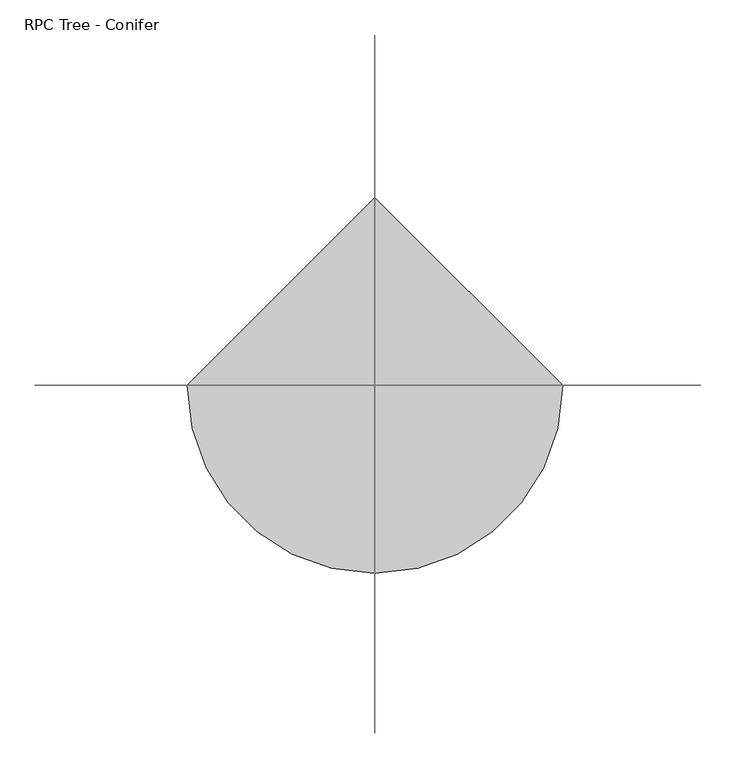
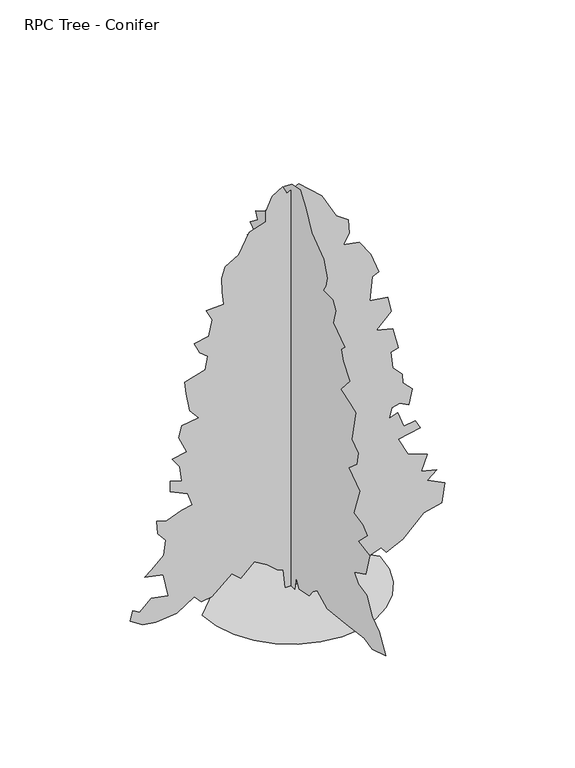
"""IFC4 building model written with IfcOpenShell, lengths in millimetres: geographic element geometry, RPC Tree - Conifer."""

from ifc_helpers import new_model, si_unit, origin, place, context, project, spatial, triangles, source, transform, mapped, element, save


def rpc_tree_conifer_9825e489(model_context):
    return source(origin(), model_context, "Body", "Tessellation", [
        triangles([(0.1966736, 56.9494036, 4.14e-05), (0.1966822, 87.893554, 239.8173931), (0.1966871, 126.5738239, 348.1206479), (0.196691, 265.8223646, 270.7615617), (0.1966966, 436.0144835, 201.1371414), (0.1967043, 629.4157963, 170.192991), (0.1967132, 823.3543219, 178.424865), (0.1967103, 846.0257578, 46.416371), (0.1967193, 985.2745983, 139.2488314), (0.196723, 1133.0273529, 41.5309043), (0.1967288, 1240.5636669, 77.3605215), (0.1967379, 1449.4382721, 69.6244157), (0.1967452, 1550.0050987, 162.4568716), (0.1967611, 1766.6151329, 371.3292603), (0.1967571, 1635.1015034, 433.2170162), (0.1967531, 1519.061348, 471.8989938), (0.1967479, 1410.9707073, 462.869276), (0.1967506, 1387.5477184, 587.9391855), (0.1967552, 1418.4916145, 696.2441299), (0.1967638, 1526.7964863, 820.0196417), (0.1967596, 1418.4916145, 843.2282541), (0.1967657, 1503.5878738, 920.5893751), (0.196761, 1372.0771511, 959.2684822), (0.1967569, 1232.8283833, 1028.8943195), (0.1967579, 1161.2365322, 1172.1522177), (0.1967675, 1341.1334003, 1222.2955959), (0.196773, 1418.4916145, 1291.9186718), (0.1967692, 1317.9247879, 1315.1272842), (0.1967646, 1147.7320513, 1415.6968723), (0.196772, 1271.5074177, 1477.5846645), (0.1967785, 1281.5201786, 1681.3043518), (0.1967728, 1139.9939335, 1701.929837), (0.1967682, 1016.2184217, 1732.8737331), (0.1967732, 1034.477845, 1873.8285015), (0.1967812, 1185.2224228, 1916.3224194), (0.196787, 1217.3549818, 2065.5239227), (0.1967808, 1093.5795427, 2042.3153103), (0.1967818, 1015.412657, 2192.8769051), (0.1967888, 1101.3147537, 2297.6043789), (0.1967867, 993.0098093, 2390.4359219), (0.1967939, 1101.3147537, 2467.7970428), (0.1967971, 1132.2586498, 2529.6848351), (0.1967921, 938.8573734, 2653.4630356), (0.1967934, 915.648761, 2730.8213951), (0.1968026, 1070.3709303, 2808.1823708), (0.1968025, 1000.745093, 2908.7634407), (0.1967977, 846.0257578, 2978.3722733), (0.1968056, 946.5925844, 3094.4151901), (0.1968038, 838.28764, 3194.9706802), (0.1968006, 699.0416336, 3295.554657), (0.1968039, 691.3035158, 3419.3415779), (0.1968107, 807.3437439, 3473.4911797), (0.1968087, 722.250246, 3535.3847855), (0.1968049, 621.6805853, 3558.5877296), (0.1968136, 753.1941422, 3651.3992157), (0.1968106, 613.9453016, 3759.7269058), (0.1968146, 652.6244087, 3837.0794518), (0.1968101, 490.1669921, 3929.9197151), (0.1968084, 358.6533989, 4069.1658669), (0.1968098, 271.8779725, 4247.7881035), (0.1968084, 111.1016033, 4440.4978523), (0.1968058, -12.6752415, 4541.0533424), (0.1967999, -167.3960687, 4572.0), (0.1967909, -275.7007406, 4432.7541389), (0.1967796, -384.0051218, 4216.1554413), (0.1967647, -608.3503306, 4053.6781494), (0.1967566, -670.2380865, 3875.7701134), (0.1967548, -639.2941904, 3767.4424232), (0.1967544, -600.6150833, 3697.8335907), (0.1967468, -770.8077473, 3697.8335907), (0.1967416, -824.9602558, 3604.9933273), (0.1967389, -778.5430309, 3442.5445221), (0.1967248, -995.1529198, 3295.554657), (0.1967261, -925.5270824, 3233.6613419), (0.1967209, -964.2090963, 3117.6181343), (0.196711, -1087.9845354, 2970.6285599), (0.1967128, -917.7918715, 2777.23862), (0.1967031, -1096.9856575, 2721.2600601), (0.1966974, -1196.2895525, 2676.6717934), (0.1966903, -1126.6636425, 2336.2834133), (0.1966826, -1242.7067047, 2251.1870087), (0.1966795, -1219.4980923, 2111.9382408), (0.1966822, -1072.5112066, 1980.4275181), (0.196669, -1273.6506008, 1841.1787502), (0.1966648, -1157.6103727, 1523.9989826), (0.1966562, -1327.8031094, 1493.0552319), (0.1966503, -1412.899514, 1423.432156), (0.1966529, -1242.7067047, 1253.239492), (0.1966423, -1459.3138321, 1222.2955959), (0.1966381, -1381.9556179, 967.0036932), (0.1966445, -1173.0808674, 866.4368666), (0.1966386, -1242.7067047, 773.6052509), (0.1966304, -1405.1613235, 742.6614275), (0.1966206, -1505.731057, 564.7305731), (0.196612, -1637.2446865, 471.8989938), (0.1966008, -1753.2848419, 270.7615617), (0.1966095, -1505.731057, 193.4010221), (0.1966173, -1353.9035511, 228.1030827), (0.1966309, -1023.5507504, 187.537154), (0.1966455, -670.2380865, 146.9846601), (0.1966566, -484.5719848, 239.8173931), (0.1966582, -407.2137706, 177.9288015), (0.1966588, -337.5878969, 92.8324604), (0.1966659, -151.9238481, 54.1524813), (0.1966712, -98.1771287, 152.3810422), (0.1966681, -66.8274934, 3.77e-05), (-58.554956, 1.5e-06, 4.14e-05), (-81.7629962, -2.37e-05, 208.8732426), (-143.6513062, -2.29e-05, 232.0812919), (-251.9559872, -2.39e-05, 324.9149059), (-391.203665, -2.35e-05, 410.0112379), (-538.1906233, 3.7e-06, 270.7615617), (-631.0222389, 2.7e-06, 355.8587657), (-847.6322004, 1.74e-05, 170.192991), (-956.4028868, 2.13e-05, 156.5801409), (-1033.295359, 1.98e-05, 239.8173931), (-1218.9614244, 3.09e-05, 116.0407913), (-1443.3066696, 5.52e-05, 92.832742), (-1582.5554375, 5.83e-05, 116.0407913), (-1714.069067, 5.84e-05, 201.1371414), (-1690.8604546, 5.29e-05, 309.4415408), (-1613.4993336, 5.27e-05, 263.0254423), (-1489.7209877, 2.72e-05, 379.0673781), (-1311.7930401, 2.33e-05, 348.1206479), (-1364.2652733, 1.34e-05, 603.6325953), (-1559.346825, 1.75e-05, 642.0916941), (-1489.7209877, 1.3e-05, 696.2441299), (-1358.210265, 3.6e-06, 820.0196417), (-1335.0016525, -4.4e-06, 982.4770947), (-1420.0980572, -6.3e-06, 1083.0468281), (-1435.571386, -1.25e-05, 1230.0308796), (-1327.2663689, -1.43e-05, 1199.0869835), (-1164.8089886, -3.85e-05, 1260.9747757), (-1056.5039715, -4.28e-05, 1284.1833881), (-1102.9211964, -4.76e-05, 1423.432156), (-1288.7501152, -4.6e-05, 1510.4659424), (-1288.5844276, -5.14e-05, 1632.3039997), (-1164.8089886, -5.34e-05, 1593.6248199), (-1185.6830051, -6.01e-05, 1758.0569344), (-1265.378722, -6.28e-05, 1872.122501), (-1110.65648, -6.88e-05, 1903.0663971), (-1195.752812, -7.46e-05, 2088.7296284), (-1164.8089886, -8.1e-05, 2212.5079742), (-986.881041, -0.0001043, 2243.4518703), (-1079.7125839, -0.0001064, 2351.7567421), (-1118.3917637, -0.0001146, 2560.6285858), (-1133.8650925, -0.00012, 2692.14207), (-917.255131, -0.0001296, 2761.7651459), (-886.3113075, -0.0001367, 2901.0197273), (-971.4076395, -0.0001373, 2970.6285599), (-1033.295359, -0.000141, 3094.4151901), (-875.9814148, -0.0001635, 3120.9042709), (-839.8940826, -0.0001723, 3295.554657), (-901.7818022, -0.000176, 3419.3415779), (-716.1185709, -0.0001819, 3427.0568047), (-731.5891382, -0.000188, 3574.0466698), (-739.3271833, -0.0001947, 3728.7802483), (-700.6452421, -0.000201, 3844.8234558), (-557.2529772, -0.0002259, 3932.9773773), (-445.3561372, -0.0002387, 4146.5181221), (-267.4279352, -0.0002465, 4200.6680145), (-267.4279352, -0.0002516, 4316.7109314), (-197.803515, -0.0002603, 4463.7007965), (-89.4991065, -0.0002666, 4533.3093384), (-43.0827355, -0.0002642, 4448.2130791), (80.6938754, -0.0002873, 4510.1066849), (328.2462433, -0.0002846, 4285.7642738), (482.9684489, -0.0002602, 4007.272261), (614.4819695, -0.0002765, 3914.4319977), (622.2172531, -0.0002533, 3759.7269058), (560.3295336, -0.0002466, 3651.3992157), (730.5221975, -0.0002503, 3620.4810448), (854.2977093, -0.000246, 3442.5445221), (939.3940413, -0.0002385, 3218.2021111), (869.0194851, -0.0002348, 3181.5976593), (838.827142, -0.0002224, 2924.2226715), (1032.2256569, -0.0002267, 2893.2760139), (1070.9075981, -0.0002203, 2723.0861115), (908.4501451, -0.0002085, 2568.3667763), (1086.3780928, -0.0002118, 2521.9495514), (1148.2687191, -0.0001863, 2282.1309048), (1063.1694803, -0.0001831, 2266.6604828), (1086.3780928, -0.0001755, 2080.9943447), (1188.6852201, -0.0001735, 1969.2404102), (1194.6831099, -0.0001693, 1872.122501), (1295.2527706, -0.0001678, 1771.5529129), (1256.5708294, -0.0001591, 1601.3601036), (1163.7392138, -0.0001587, 1655.5126122), (1078.6428818, -0.0001552, 1632.3039997), (1047.6989857, -0.0001494, 1523.9989826), (1140.5306013, -0.0001535, 1554.9428787), (1202.4183208, -0.0001474, 1377.0149311), (1326.1966667, -0.0001522, 1400.2235435), (1380.3491753, -0.0001493, 1299.6538101), (1148.2687191, -0.0001403, 1253.239492), (1248.8355457, -0.0001177, 1052.1000978), (1457.7102962, -0.0001371, 974.741811), (1390.8704807, -0.0001109, 804.5519812), (1558.2771229, -0.0001141, 765.8671331), (1457.7102962, -0.0001073, 680.7708012), (1643.3733822, -0.0001087, 587.9391855), (1612.4296314, -9.81e-05, 371.3292603), (1419.0282097, -9.03e-05, 324.9149059), (1195.7460537, -7.39e-05, 107.7223219), (1016.7551622, -4.82e-05, 23.2080424), (962.6026537, -4.97e-05, 92.8324604), (759.5372869, -4.06e-05, 23.9482793), (544.8561685, -3.38e-05, 15.472048), (459.7598365, -3.47e-05, 92.8324604), (266.3587781, -3.2e-05, 162.4568716), (83.8288403, -2.49e-05, 125.065631), (65.2216548, -1.88e-05, 3.77e-05), (-946.6959938, -5.2e-06, 6.79e-05), (-921.6614027, -216.9648272, 6.07e-05), (-850.3696787, -416.2120222, 5.26e-05), (-738.5242527, -592.0339937, 4.4e-05), (-591.8373124, -738.7208977, 3.53e-05), (-416.0153409, -850.5663237, 2.67e-05), (-216.7681641, -921.8580477, 1.87e-05), (0.1967125, -946.8926388, 1.14e-05), (217.1614903, -921.8580477, 5.7e-06), (416.4087035, -850.5663237, 1.9e-06), (592.230675, -738.7208977, 0.0), (738.9175426, -592.0339937, 0.0), (850.7629686, -416.2120222, 1.9e-06), (922.0546926, -216.9648272, 5.7e-06), (947.0892838, 8.77e-05, 1.14e-05), (0.1965469, 946.8926388, 6.79e-05)], [[26, 27, 28], [21, 22, 23], [19, 20, 21], [51, 52, 53], [7, 8, 9], [35, 36, 37], [13, 14, 15], [34, 35, 37], [54, 55, 56], [72, 73, 74], [95, 96, 97], [88, 89, 90], [44, 45, 46], [86, 87, 88], [85, 86, 88], [51, 53, 54], [44, 46, 47], [88, 90, 91], [13, 15, 16], [13, 16, 17], [38, 39, 40], [25, 26, 28], [25, 28, 29], [47, 48, 49], [56, 57, 58], [30, 31, 32], [29, 30, 32], [41, 42, 43], [40, 41, 43], [106, 1, 2], [105, 106, 2], [75, 76, 77], [94, 95, 97], [94, 97, 98], [78, 79, 80], [83, 84, 85], [29, 32, 33], [103, 104, 105], [12, 13, 17], [11, 12, 17], [77, 78, 80], [102, 103, 105], [62, 63, 64], [80, 81, 82], [80, 82, 83], [61, 62, 64], [61, 64, 65], [60, 61, 65], [59, 60, 65], [69, 70, 71], [69, 71, 72], [94, 98, 99], [93, 94, 99], [92, 93, 99], [92, 99, 100], [91, 92, 100], [91, 100, 101], [47, 49, 50], [9, 10, 11], [9, 11, 17], [9, 17, 18], [7, 9, 18], [59, 65, 66], [59, 66, 67], [59, 67, 68], [59, 68, 69], [58, 59, 69], [56, 58, 69], [54, 56, 69], [54, 69, 72], [51, 54, 72], [50, 51, 72], [50, 72, 74], [50, 74, 75], [50, 75, 77], [47, 50, 77], [44, 47, 77], [43, 44, 77], [40, 43, 77], [40, 77, 80], [40, 80, 83], [38, 40, 83], [38, 83, 85], [37, 38, 85], [34, 37, 85], [33, 34, 85], [29, 33, 85], [25, 29, 85], [25, 85, 88], [25, 88, 91], [25, 91, 101], [25, 101, 102], [24, 25, 102], [23, 24, 102], [21, 23, 102], [105, 2, 3], [102, 105, 3], [21, 102, 3], [21, 3, 4], [21, 4, 5], [21, 5, 6], [21, 6, 7], [21, 7, 18], [19, 21, 18], [125, 126, 127], [198, 199, 200], [153, 154, 155], [139, 140, 141], [130, 131, 132], [120, 121, 122], [119, 120, 122], [186, 187, 188], [136, 137, 138], [135, 136, 138], [150, 151, 152], [193, 194, 195], [192, 193, 195], [125, 127, 128], [180, 181, 182], [163, 164, 165], [185, 186, 188], [196, 197, 198], [190, 191, 192], [111, 112, 113], [212, 107, 108], [211, 212, 108], [173, 174, 175], [149, 150, 152], [179, 180, 182], [129, 130, 132], [146, 147, 148], [204, 205, 206], [200, 201, 202], [200, 202, 203], [162, 163, 165], [190, 192, 195], [165, 166, 167], [118, 119, 122], [118, 122, 123], [118, 123, 124], [117, 118, 124], [116, 117, 124], [176, 177, 178], [176, 178, 179], [129, 132, 133], [185, 188, 189], [142, 143, 144], [141, 142, 144], [161, 162, 165], [161, 165, 167], [161, 167, 168], [116, 124, 125], [145, 146, 148], [144, 145, 148], [114, 115, 116], [113, 114, 116], [113, 116, 125], [113, 125, 128], [113, 128, 129], [113, 129, 133], [113, 133, 134], [111, 113, 134], [168, 169, 170], [168, 170, 171], [161, 168, 171], [160, 161, 171], [159, 160, 171], [158, 159, 171], [157, 158, 171], [156, 157, 171], [155, 156, 171], [171, 172, 173], [171, 173, 175], [155, 171, 175], [155, 175, 176], [153, 155, 176], [152, 153, 176], [149, 152, 176], [149, 176, 179], [148, 149, 179], [144, 148, 179], [144, 179, 182], [144, 182, 183], [141, 144, 183], [139, 141, 183], [138, 139, 183], [135, 138, 183], [134, 135, 183], [111, 134, 183], [110, 111, 183], [110, 183, 184], [110, 184, 185], [110, 185, 189], [110, 189, 190], [110, 190, 195], [109, 110, 195], [108, 109, 195], [211, 108, 195], [210, 211, 195], [210, 195, 196], [209, 210, 196], [209, 196, 198], [208, 209, 198], [207, 208, 198], [206, 207, 198], [204, 206, 198], [203, 204, 198], [200, 203, 198], [227, 228, 213], [226, 227, 213], [226, 213, 214], [225, 226, 214], [225, 214, 215], [225, 215, 216], [224, 225, 216], [223, 224, 216], [223, 216, 217], [223, 217, 218], [223, 218, 219], [223, 219, 220], [223, 220, 221], [223, 221, 222]], closed=False),
    ])


if __name__ == "__main__":
    model = new_model("IFC4")
    model_context = context("Model", 3, world=origin())
    ifc_project = project(units=[si_unit("LENGTHUNIT", "METRE", prefix="MILLI")], contexts=[model_context])
    site = spatial("IfcSite", under=ifc_project)
    building = spatial("IfcBuilding", under=site)
    placement = place(None, origin())
    rpc_tree_conifer_shape = rpc_tree_conifer_9825e489(model_context)
    element("IfcGeographicElement", 1, ObjectType="RPC Tree - Conifer", at=placement, inside=building, context=model_context, shape_type="MappedRepresentation", body=[
        mapped(rpc_tree_conifer_shape, transform((0.0, 0.0, 0.0), x_axis=(1.0, 0.0, 0.0), y_axis=(0.0, 1.0, 0.0), z_axis=(0.0, 0.0, 1.0))),
    ])
    save(model, "model.ifc")

# Revit data of these elements
# Type "RPC Tree - Conifer"
#   built-in parameter 1005198 = "{2, 15},{39, RPC-16-G0M4-N9PX-U6TN-C000-ST1L-LVER-AU},{1, 0},{1, 0},{2, 35},{1, 8},{5, Color},{1, 0},{1, 0},{3, 0.8},{3, 0.8},{3, 0.8},{1, 8},{7, BBoxMin},{1, 0},{1, 0},{1, 0},{1, 0},{1, 0},{1, 8},{7, BBoxMax},{1, 0},{1, 0},{1, 0},{1, 0},{1, 0},{2, 11},{9, RPCTypeId},{1, 0},{1, 0},{39, RPC-16-G0M4-N9PX-U6TN-C000-ST1L-LVER-AU},{1, 6},{14, RPCPlantHeight},{1, 0},{1, 0},{2, 13},{2, 11},{7, keyword},{1, 0},{1, 0},{91, :Geometry:RPC:Colorado Spruce:colorado spruce:pinaceae:picea:pungens:evergreen:conifer:blue},{2, 11},{8, category},{1, 0},{1, 0},{16, :Trees [General]},{2, 11},{12, LocalizedUID},{1, 0},{1, 0},{15, Colorado Spruce},{2, 14},{6, Height},{1, 0},{1, 0},{2, 13},{1, 2},{16, Cast Reflections},{1, 0},{1, 0},{1, 0},{1, 2},{12, Cast Shadows},{1, 0},{1, 0},{1, 1},{1, 2},{9, Lock View},{1, 0},{1, 0},{1, 0},{1, 4},{5, ViewC},{1, 0},{1, 0},{1, 0},{2, 11},{20, AdvancedUIDefinition},{1, 0},{1, 0},{0, },{2, 11},{10, AssetLibID},{1, 0},{1, 0},{36, 4D3F6E72-3F99-4203-98E9-AF80B3C7A7A4},{2, 11},{10, BaseSchema},{1, 0},{1, 0},{9, RPCSchema},{2, 11},{12, ExchangeGUID},{1, 0},{1, 0},{0, },{1, 2},{6, Hidden},{1, 0},{1, 0},{1, 0},{1, 4},{11, RPCCategory},{1, 0},{1, 0},{1, 0},{2, 11},{8, RPCImage},{1, 0},{1, 0},{0, },{1, 4},{13, SchemaVersion},{1, 0},{1, 0},{1, 4},{2, 11},{12, UIDefinition},{1, 0},{1, 0},{0, },{2, 11},{6, UIName},{1, 0},{1, 0},{39, RPC-16-G0M4-N9PX-U6TN-C000-ST1L-LVER-AU},{2, 11},{11, VersionGUID},{1, 0},{1, 0},{9, RPCSchema},{2, 11},{9, assettype},{1, 0},{1, 0},{11, RPCGeometry},{2, 11},{11, description},{1, 0},{1, 0},{0, },{2, 11},{9, localname},{1, 0},{1, 0},{3, RPC},{2, 11},{9, localtype},{1, 0},{1, 0},{3, RPC},{1, 4},{8, revision},{1, 0},{1, 0},{1, 1},{2, 11},{9, thumbnail},{1, 0},{1, 0},{0, },{1, 4},{7, version},{1, 0},{1, 0},{1, 1},{1, 2},{20, RPC_Cast Reflections},{1, 0},{1, 0},{1, 1},{1, 2},{16, RPC_Cast Shadows},{1, 0},{1, 0},{1, 1},{1, 2},{13, RPC_Lock View},{1, 0},{1, 0},{1, 0},{1, 4},{9, RPC_ViewC},{1, 0},{1, 0},{1, 0},{21, assetlibrary_base.fbx},{1, 5},"
#   built-in parameter 1005195 = "RPC-16-G0M4-N9PX-U6TN-C000-ST1L-LVER-AU"
#   Assembly Code = "G2050500"
#   Height = 15' - 0"
#   Description = (empty or 0)
#   Default Elevation = 0
